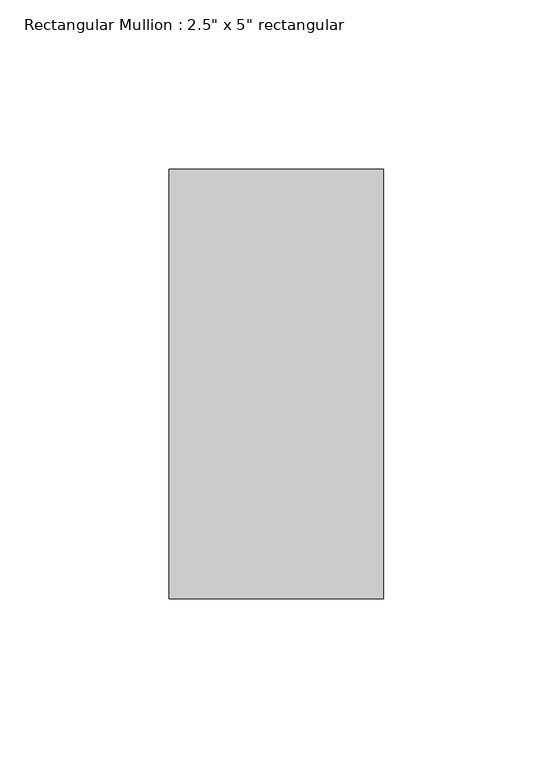
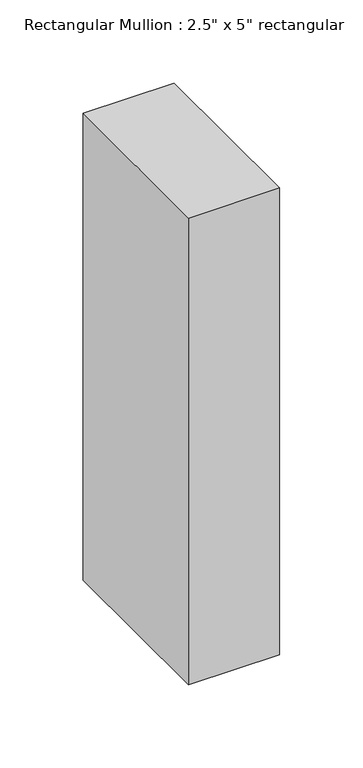
"""IFC4 building model written with IfcOpenShell, lengths in millimetres: member geometry."""

from ifc_helpers import new_model, si_unit, frame, origin, place, context, project, spatial, polyline, outline, extrude, source, transform, mapped, element, save


def member_5aeb4b7d(model_context):
    return source(origin(), model_context, "Body", "SweptSolid", [
        extrude(outline(polyline([(31.75, 63.5), (31.75, -63.5), (-31.75, -63.5), (-31.75, 63.5), (31.75, 63.5)])), frame((0.0, 0.0, -342.9), z_axis=(0.0, 0.0, 1.0), x_axis=(1.0, 0.0, 0.0)), (0.0, 0.0, 1.0), 342.9),
    ])


if __name__ == "__main__":
    model = new_model("IFC4")
    model_context = context("Model", 3, world=origin())
    ifc_project = project(units=[si_unit("LENGTHUNIT", "METRE", prefix="MILLI")], contexts=[model_context])
    site = spatial("IfcSite", under=ifc_project)
    building = spatial("IfcBuilding", under=site)
    placement = place(None, origin())
    member_shape = member_5aeb4b7d(model_context)
    element("IfcMember", 1, ObjectType="Rectangular Mullion : 2.5\" x 5\" rectangular", at=placement, inside=building, context=model_context, shape_type="MappedRepresentation", body=[
        mapped(member_shape, transform((0.0, 0.0, 0.0), x_axis=(1.0, 0.0, 0.0), y_axis=(0.0, 1.0, 0.0), z_axis=(0.0, 0.0, 1.0))),
    ])
    save(model, "model.ifc")

# Revit data of these elements
# Type "Rectangular Mullion : 2.5\" x 5\" rectangular"
#   built-in parameter 1007304 = 0.416667 (stored number, unit not read)
#   built-in parameter 1007301 = 0.104167 (stored number, unit not read)
#   built-in parameter 1007300 = 0.104167 (stored number, unit not read)
# Element 1 (IfcMember, "Rectangular Mullion : 2.5\" x 5\" rectangular")
#   Materials on its faces: "Aluminum"
# Materials
#   "Aluminum": class "Metal", colour RGB 247 247 247, transparency 0, Description = "Aluminum 6061", Cost = 0
